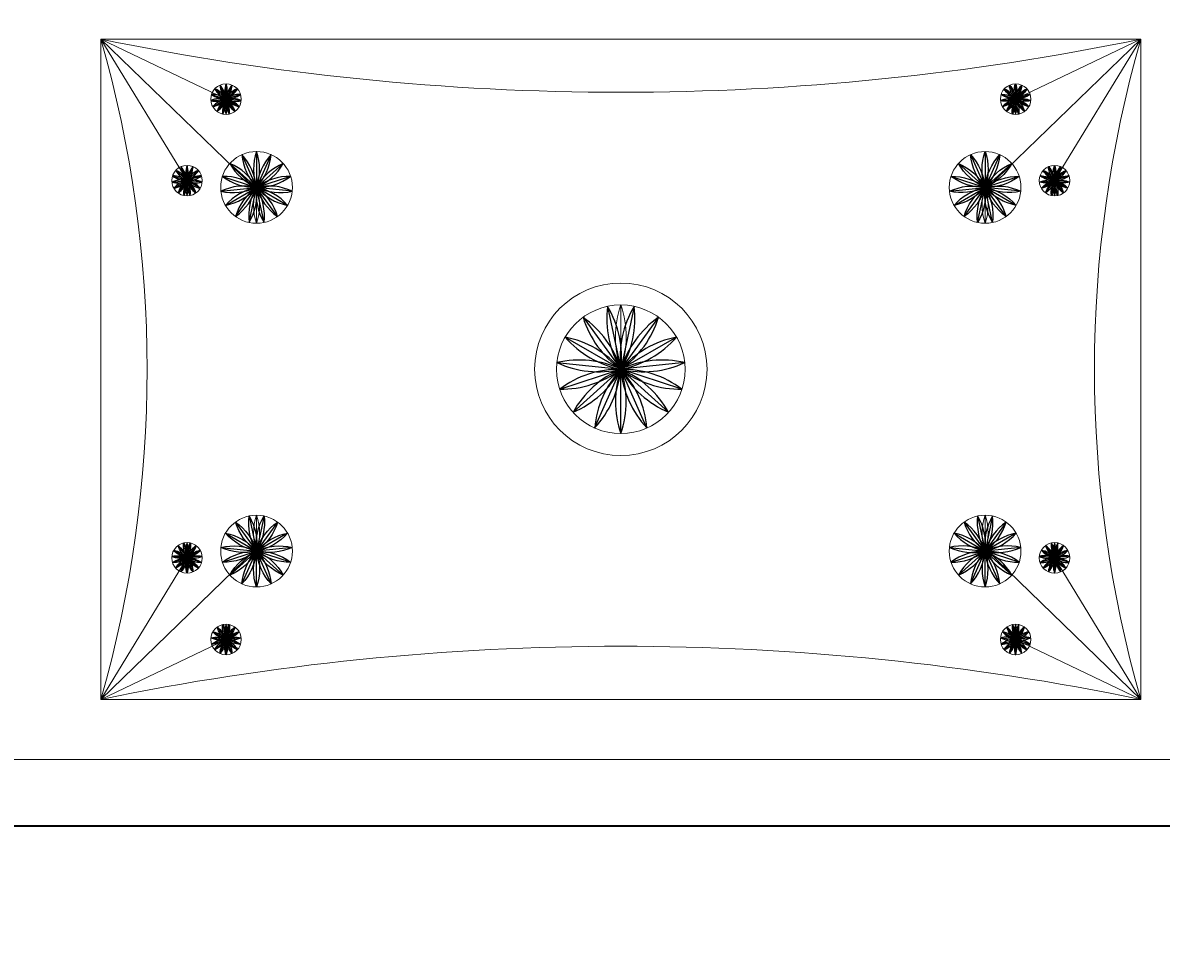
# Model space of a CAD drawing. Units: inches. Extents: x -61 to 1599, y -1316 to 257.
# Tile 117 of 204: x 134 to 161, y -10 to 11. Entities that reach past the tile are written whole.
import ezdxf

# ---------------------------------------------------------------- set-up
doc = ezdxf.new("R2010")
doc.units = ezdxf.units.IN
doc.header["$MEASUREMENT"] = 0
for name, color, linetype, lineweight in [('A-ANNO-DIMS', 2, 'Continuous', 18), ('FURNITURE', 83, 'Continuous', 18), ('WALLS', 4, 'Continuous', 35)]:
    doc.layers.add(name, color=color, linetype=linetype, lineweight=lineweight)
doc.layers.add('LT', color=8, linetype='Continuous')
doc.styles.get("Standard").update_dxf_attribs({"font": 'arial.ttf'})
doc.dimstyles.get("Standard").update_dxf_attribs({"dimtxt": 0.18, "dimasz": 0.18, "dimexe": 0.18, "dimexo": 0.0625, "dimgap": 0.09, "dimtad": 0, "dimtih": 1, "dimtoh": 1, "dimdec": 0, "dimzin": 0, "dimdsep": 46, "dimlunit": 3, "dimtxsty": 'Standard', "dimcen": 0.09, "dimadec": 0, "dimazin": 0, "dimtfac": 1, "dimtdec": 0, "dimtofl": 0, "dimtmove": 0, "dimatfit": 3, "dimfxl": 1, "dimtolj": 1, "dimtzin": 0, "dimarcsym": 0})

# ---------------------------------------------------------------- blocks, each defined once
blk = doc.blocks.new('*U3')
at = {"layer": 'LT'}
blk.add_line((0, 0.175), (0, -0.175), dxfattribs=at)
for centre, start, end in [((0.509, 0), 160.9983, 199.0017), ((-0.509, 0), 340.9983, 19.0017)]:
    blk.add_arc(centre, 0.539, start, end, dxfattribs=at)
blk = doc.blocks.new('*U4')
at = {"layer": 'LT', "transparency": 16777216}
for p, rotation in [((-66.605, -18.692), 48.00000000000001), ((-66.546, -18.649), 24), ((-66.404, -18.649), 336.0000000000001), ((-66.345, -18.692), 312), ((-66.649, -18.828), 96), ((-66.642, -18.755), 72), ((-66.627, -18.897), 120), ((-66.578, -18.951), 144), ((-66.512, -18.981), 168.0000000000001), ((-66.439, -18.981), 192), ((-66.372, -18.951), 216), ((-66.323, -18.897), 240), ((-66.308, -18.755), 288.0000000000001), ((-66.301, -18.828), 264)]:
    blk.add_blockref('*U3', p, dxfattribs=dict(at, rotation=rotation))
blk.add_blockref('*U3', (-66.475, -18.634), dxfattribs=at)
blk = doc.blocks.new('*U20')
at = {"layer": 'LT'}
blk.add_line((0, 0.175), (0, -0.175), dxfattribs=at)
for centre, start, end in [((0.509, 0), 160.9983, 199.0017), ((-0.509, 0), 340.9983, 19.0017)]:
    blk.add_arc(centre, 0.539, start, end, dxfattribs=at)
blk = doc.blocks.new('*U21')
at = {"layer": 'LT', "transparency": 16777216}
for p, rotation in [((-66.605, -18.692), 48.00000000000001), ((-66.546, -18.649), 24), ((-66.404, -18.649), 336.0000000000001), ((-66.345, -18.692), 312), ((-66.649, -18.828), 96), ((-66.642, -18.755), 72), ((-66.627, -18.897), 120), ((-66.578, -18.951), 144), ((-66.512, -18.981), 168.0000000000001), ((-66.439, -18.981), 192), ((-66.372, -18.951), 216), ((-66.323, -18.897), 240), ((-66.308, -18.755), 288.0000000000001), ((-66.301, -18.828), 264)]:
    blk.add_blockref('*U20', p, dxfattribs=dict(at, rotation=rotation))
blk.add_blockref('*U20', (-66.475, -18.634), dxfattribs=at)
blk = doc.blocks.new('*U52')
at = {"layer": 'LT'}
blk.add_line((0, 0.175), (0, -0.175), dxfattribs=at)
for centre, start, end in [((0.509, 0), 160.9983, 199.0017), ((-0.509, 0), 340.9983, 19.0017)]:
    blk.add_arc(centre, 0.539, start, end, dxfattribs=at)
blk = doc.blocks.new('*U53')
at = {"layer": 'LT', "transparency": 16777216}
for p, rotation in [((-66.605, -18.692), 48.00000000000001), ((-66.546, -18.649), 24), ((-66.404, -18.649), 336.0000000000001), ((-66.345, -18.692), 312), ((-66.649, -18.828), 96), ((-66.642, -18.755), 72), ((-66.627, -18.897), 120), ((-66.578, -18.951), 144), ((-66.512, -18.981), 168.0000000000001), ((-66.439, -18.981), 192), ((-66.372, -18.951), 216), ((-66.323, -18.897), 240), ((-66.308, -18.755), 288.0000000000001), ((-66.301, -18.828), 264)]:
    blk.add_blockref('*U52', p, dxfattribs=dict(at, rotation=rotation))
blk.add_blockref('*U52', (-66.475, -18.634), dxfattribs=at)
blk = doc.blocks.new('*U29')
at = {"layer": 'LT'}
blk.add_line((0, 0.175), (0, -0.175), dxfattribs=at)
for centre, start, end in [((0.509, 0), 160.9983, 199.0017), ((-0.509, 0), 340.9983, 19.0017)]:
    blk.add_arc(centre, 0.539, start, end, dxfattribs=at)
blk = doc.blocks.new('*U30')
at = {"layer": 'LT', "transparency": 16777216}
for p, rotation in [((-66.605, -18.692), 48.00000000000001), ((-66.546, -18.649), 24), ((-66.404, -18.649), 336.0000000000001), ((-66.345, -18.692), 312), ((-66.649, -18.828), 96), ((-66.642, -18.755), 72), ((-66.627, -18.897), 120), ((-66.578, -18.951), 144), ((-66.512, -18.981), 168.0000000000001), ((-66.439, -18.981), 192), ((-66.372, -18.951), 216), ((-66.323, -18.897), 240), ((-66.308, -18.755), 288.0000000000001), ((-66.301, -18.828), 264)]:
    blk.add_blockref('*U29', p, dxfattribs=dict(at, rotation=rotation))
blk.add_blockref('*U29', (-66.475, -18.634), dxfattribs=at)
blk = doc.blocks.new('*U5')
at = {"layer": 'LT'}
blk.add_line((0, 0.412), (0, -0.412), dxfattribs=at)
for centre, start, end in [((1.198, 0), 160.9983, 199.0017), ((-1.198, 0), 340.9983, 19.0017)]:
    blk.add_arc(centre, 1.267, start, end, dxfattribs=at)
blk = doc.blocks.new('*U47')
at = {"layer": 'LT', "transparency": 16777216}
for p, rotation in [((-156.501, -43.858), 24), ((-156.165, -43.858), 336.0000000000001), ((-156.639, -43.959), 48.00000000000001), ((-156.027, -43.959), 312), ((-156.725, -44.108), 72), ((-155.941, -44.108), 288.0000000000001), ((-156.743, -44.278), 96), ((-156.69, -44.441), 120), ((-156.575, -44.569), 144), ((-156.419, -44.639), 168), ((-156.247, -44.639), 192), ((-156.091, -44.569), 216), ((-155.976, -44.441), 240), ((-155.923, -44.278), 264)]:
    blk.add_blockref('*U5', p, dxfattribs=dict(at, rotation=rotation))
blk.add_blockref('*U5', (-156.333, -43.823), dxfattribs=at)
blk = doc.blocks.new('*U22')
at = {"layer": 'LT'}
blk.add_line((0, 0.412), (0, -0.412), dxfattribs=at)
for centre, start, end in [((1.198, 0), 160.9983, 199.0017), ((-1.198, 0), 340.9983, 19.0017)]:
    blk.add_arc(centre, 1.267, start, end, dxfattribs=at)
blk = doc.blocks.new('*U23')
at = {"layer": 'LT', "transparency": 16777216}
for p, rotation in [((-156.501, -43.858), 24), ((-156.165, -43.858), 336.0000000000001), ((-156.639, -43.959), 48.00000000000001), ((-156.027, -43.959), 312), ((-156.725, -44.108), 72), ((-155.941, -44.108), 288.0000000000001), ((-156.743, -44.278), 96), ((-156.69, -44.441), 120), ((-156.575, -44.569), 144), ((-156.419, -44.639), 168), ((-156.247, -44.639), 192), ((-156.091, -44.569), 216), ((-155.976, -44.441), 240), ((-155.923, -44.278), 264)]:
    blk.add_blockref('*U22', p, dxfattribs=dict(at, rotation=rotation))
blk.add_blockref('*U22', (-156.333, -43.823), dxfattribs=at)
blk = doc.blocks.new('*U54')
at = {"layer": 'LT'}
blk.add_line((0, 0.739), (0, -0.739), dxfattribs=at)
for centre, start, end in [((2.147, 0), 160.9983, 199.0017), ((-2.147, 0), 340.9983, 19.0017)]:
    blk.add_arc(centre, 2.27, start, end, dxfattribs=at)
blk = doc.blocks.new('*U41')
at = {"layer": 'LT', "transparency": 16777216}
for p, rotation in [((-280.542, -78.621), 23.99999999999999), ((-279.941, -78.621), 336.0000000000001), ((-280.791, -78.801), 48.00000000000001), ((-279.692, -78.801), 312), ((-280.945, -79.067), 72), ((-279.539, -79.067), 288.0000000000001), ((-280.977, -79.373), 96), ((-280.882, -79.665), 120), ((-280.676, -79.894), 144), ((-280.395, -80.019), 168), ((-280.088, -80.019), 191.9999999999999), ((-279.807, -79.894), 216), ((-279.602, -79.665), 240), ((-279.507, -79.373), 264)]:
    blk.add_blockref('*U54', p, dxfattribs=dict(at, rotation=rotation))
blk.add_blockref('*U54', (-280.242, -78.557), dxfattribs=at)
blk = doc.blocks.new('*U42')
at = {"layer": 'LT'}
blk.add_line((0, 0.412), (0, -0.412), dxfattribs=at)
for centre, start, end in [((1.198, 0), 160.9983, 199.0017), ((-1.198, 0), 340.9983, 19.0017)]:
    blk.add_arc(centre, 1.267, start, end, dxfattribs=at)
blk = doc.blocks.new('*U43')
at = {"layer": 'LT', "transparency": 16777216}
for p, rotation in [((-156.501, -43.858), 24), ((-156.165, -43.858), 336.0000000000001), ((-156.639, -43.959), 48.00000000000001), ((-156.027, -43.959), 312), ((-156.725, -44.108), 72), ((-155.941, -44.108), 288.0000000000001), ((-156.743, -44.278), 96), ((-156.69, -44.441), 120), ((-156.575, -44.569), 144), ((-156.419, -44.639), 168), ((-156.247, -44.639), 192), ((-156.091, -44.569), 216), ((-155.976, -44.441), 240), ((-155.923, -44.278), 264)]:
    blk.add_blockref('*U42', p, dxfattribs=dict(at, rotation=rotation))
blk.add_blockref('*U42', (-156.333, -43.823), dxfattribs=at)
blk = doc.blocks.new('*U31')
at = {"layer": 'LT'}
blk.add_line((0, 0.412), (0, -0.412), dxfattribs=at)
for centre, start, end in [((1.198, 0), 160.9983, 199.0017), ((-1.198, 0), 340.9983, 19.0017)]:
    blk.add_arc(centre, 1.267, start, end, dxfattribs=at)
blk = doc.blocks.new('*U32')
at = {"layer": 'LT', "transparency": 16777216}
for p, rotation in [((-156.501, -43.858), 24), ((-156.165, -43.858), 336.0000000000001), ((-156.639, -43.959), 48.00000000000001), ((-156.027, -43.959), 312), ((-156.725, -44.108), 72), ((-155.941, -44.108), 288.0000000000001), ((-156.743, -44.278), 96), ((-156.69, -44.441), 120), ((-156.575, -44.569), 144), ((-156.419, -44.639), 168), ((-156.247, -44.639), 192), ((-156.091, -44.569), 216), ((-155.976, -44.441), 240), ((-155.923, -44.278), 264)]:
    blk.add_blockref('*U31', p, dxfattribs=dict(at, rotation=rotation))
blk.add_blockref('*U31', (-156.333, -43.823), dxfattribs=at)
blk = doc.blocks.new('*U48')
at = {"layer": 'LT'}
blk.add_line((0, 0.175), (0, -0.175), dxfattribs=at)
for centre, start, end in [((0.509, 0), 160.9983, 199.0017), ((-0.509, 0), 340.9983, 19.0017)]:
    blk.add_arc(centre, 0.539, start, end, dxfattribs=at)
blk = doc.blocks.new('*U49')
at = {"layer": 'LT', "transparency": 16777216}
for p, rotation in [((-66.605, -18.692), 48.00000000000001), ((-66.546, -18.649), 24), ((-66.404, -18.649), 336.0000000000001), ((-66.345, -18.692), 312), ((-66.649, -18.828), 96), ((-66.642, -18.755), 72), ((-66.627, -18.897), 120), ((-66.578, -18.951), 144), ((-66.512, -18.981), 168.0000000000001), ((-66.439, -18.981), 192), ((-66.372, -18.951), 216), ((-66.323, -18.897), 240), ((-66.308, -18.755), 288.0000000000001), ((-66.301, -18.828), 264)]:
    blk.add_blockref('*U48', p, dxfattribs=dict(at, rotation=rotation))
blk.add_blockref('*U48', (-66.475, -18.634), dxfattribs=at)
blk = doc.blocks.new('*U24')
at = {"layer": 'LT'}
blk.add_line((0, 0.175), (0, -0.175), dxfattribs=at)
for centre, start, end in [((0.509, 0), 160.9983, 199.0017), ((-0.509, 0), 340.9983, 19.0017)]:
    blk.add_arc(centre, 0.539, start, end, dxfattribs=at)
blk = doc.blocks.new('*U25')
at = {"layer": 'LT', "transparency": 16777216}
for p, rotation in [((-66.605, -18.692), 48.00000000000001), ((-66.546, -18.649), 24), ((-66.404, -18.649), 336.0000000000001), ((-66.345, -18.692), 312), ((-66.649, -18.828), 96), ((-66.642, -18.755), 72), ((-66.627, -18.897), 120), ((-66.578, -18.951), 144), ((-66.512, -18.981), 168.0000000000001), ((-66.439, -18.981), 192), ((-66.372, -18.951), 216), ((-66.323, -18.897), 240), ((-66.308, -18.755), 288.0000000000001), ((-66.301, -18.828), 264)]:
    blk.add_blockref('*U24', p, dxfattribs=dict(at, rotation=rotation))
blk.add_blockref('*U24', (-66.475, -18.634), dxfattribs=at)
blk = doc.blocks.new('*U50')
at = {"layer": 'LT'}
blk.add_line((0, 0.175), (0, -0.175), dxfattribs=at)
for centre, start, end in [((0.509, 0), 160.9983, 199.0017), ((-0.509, 0), 340.9983, 19.0017)]:
    blk.add_arc(centre, 0.539, start, end, dxfattribs=at)
blk = doc.blocks.new('*U51')
at = {"layer": 'LT', "transparency": 16777216}
for p, rotation in [((-66.605, -18.692), 48.00000000000001), ((-66.546, -18.649), 24), ((-66.404, -18.649), 336.0000000000001), ((-66.345, -18.692), 312), ((-66.649, -18.828), 96), ((-66.642, -18.755), 72), ((-66.627, -18.897), 120), ((-66.578, -18.951), 144), ((-66.512, -18.981), 168.0000000000001), ((-66.439, -18.981), 192), ((-66.372, -18.951), 216), ((-66.323, -18.897), 240), ((-66.308, -18.755), 288.0000000000001), ((-66.301, -18.828), 264)]:
    blk.add_blockref('*U50', p, dxfattribs=dict(at, rotation=rotation))
blk.add_blockref('*U50', (-66.475, -18.634), dxfattribs=at)
blk = doc.blocks.new('*U26')
at = {"layer": 'LT'}
blk.add_line((0, 0.175), (0, -0.175), dxfattribs=at)
for centre, start, end in [((0.509, 0), 160.9983, 199.0017), ((-0.509, 0), 340.9983, 19.0017)]:
    blk.add_arc(centre, 0.539, start, end, dxfattribs=at)
blk = doc.blocks.new('*U27')
at = {"layer": 'LT', "transparency": 16777216}
for p, rotation in [((-66.605, -18.692), 48.00000000000001), ((-66.546, -18.649), 24), ((-66.404, -18.649), 336.0000000000001), ((-66.345, -18.692), 312), ((-66.649, -18.828), 96), ((-66.642, -18.755), 72), ((-66.627, -18.897), 120), ((-66.578, -18.951), 144), ((-66.512, -18.981), 168.0000000000001), ((-66.439, -18.981), 192), ((-66.372, -18.951), 216), ((-66.323, -18.897), 240), ((-66.308, -18.755), 288.0000000000001), ((-66.301, -18.828), 264)]:
    blk.add_blockref('*U26', p, dxfattribs=dict(at, rotation=rotation))
blk.add_blockref('*U26', (-66.475, -18.634), dxfattribs=at)
blk = doc.blocks.new('BED-DOUBLE')
for p, q in [((37.147, 1.379), (37.147, 16.557)), ((61.064, 16.557), (37.147, 16.557)), ((37.147, 16.557), (40.027, 15.18)), ((37.147, 16.557), (40.715, 13.107)), ((37.147, 16.557), (39.13, 13.305)), ((61.064, 16.557), (57.496, 13.107)), ((61.064, 16.557), (58.185, 15.18)), ((61.064, 16.557), (59.081, 13.305)), ((40.027, 15.18), (40.027, 14.829)), ((58.185, 15.18), (58.185, 14.829)), ((39.13, 13.305), (39.13, 12.955)), ((40.729, 13.149), (40.729, 12.324)), ((57.483, 13.149), (57.483, 12.324)), ((59.081, 13.305), (59.081, 12.955)), ((49.106, 8.968), (49.106, 10.447)), ((40.729, 4.788), (40.729, 5.613)), ((57.483, 4.788), (57.483, 5.613)), ((39.13, 4.631), (39.13, 4.982)), ((59.081, 4.631), (59.081, 4.982)), ((37.147, 1.379), (40.715, 4.83)), ((61.064, 1.379), (57.496, 4.83)), ((37.147, 1.379), (39.13, 4.631)), ((61.064, 1.379), (59.081, 4.631)), ((40.027, 2.756), (40.027, 3.107)), ((58.185, 2.756), (58.185, 3.107)), ((37.147, 1.379), (40.027, 2.756)), ((61.064, 1.379), (58.185, 2.756)), ((61.064, 1.379), (61.064, 1.379))]:
    blk.add_line(p, q)
for points in [[(1.272, 88.537), (1.272, 3.449, 0.414214), (4.722, 0), (66.813, 0, 0.414214), (70.263, 3.449), (70.263, 88.537, 0.414214), (66.813, 91.987), (4.722, 91.987, 0.414214)], [(40.027, 15.18, 0.167358), (40.027, 14.829, 0.167358)], [(39.13, 13.305, 0.167358), (39.13, 12.955, 0.167358)], [(40.729, 13.149, 0.167358), (40.729, 12.324, 0.167358)], [(57.483, 12.324, 0.167358), (57.483, 13.149, 0.167358)], [(59.081, 12.955, 0.167358), (59.081, 13.305, 0.167358)], [(49.106, 8.968, 0.167358), (49.106, 10.447, 0.167358)], [(40.729, 5.613, 0.167358), (40.729, 4.788, 0.167358)], [(57.483, 4.788, 0.167358), (57.483, 5.613, 0.167358)], [(39.13, 4.982, 0.167358), (39.13, 4.631, 0.167358)], [(59.081, 4.631, 0.167358), (59.081, 4.982, 0.167358)], [(40.027, 3.107, 0.167358), (40.027, 2.756, 0.167358)], [(58.185, 2.756, 0.167358), (58.185, 3.107, 0.167358)]]:
    blk.add_lwpolyline(points, format="xyb", close=True)
blk.add_lwpolyline([(61.064, 16.557), (61.064, 1.379), (37.147, 1.379)])
for centre, radius in [((40.027, 15.18), 0.351), ((58.185, 15.18), 0.351), ((40.729, 13.149), 0.825), ((57.483, 13.149), 0.825), ((39.13, 13.305), 0.351), ((59.081, 13.305), 0.351), ((49.106, 8.968), 1.982), ((49.106, 8.968), 1.478), ((40.729, 4.788), 0.825), ((57.483, 4.788), 0.825), ((39.13, 4.631), 0.351), ((59.081, 4.631), 0.351), ((40.027, 2.756), 0.351), ((58.185, 2.756), 0.351)]:
    blk.add_circle(centre, radius)
for centre, radius, start, end in [((10.674, 8.968), 27.54, 344.0046, 15.9954), ((49.106, 74.54), 59.203, 258.34678, 281.65322), ((87.538, 8.968), 27.54, 164.0046, 195.9954), ((58.694, 15.005), 0.539, 160.9983, 199.0017), ((57.675, 15.005), 0.539, 340.9983, 19.0017), ((49.106, -56.603), 59.203, 78.34678, 101.65322)]:
    blk.add_arc(centre, radius, start, end)
for name, p in [('*U30', (106.502, 33.99)), ('*U23', (197.062, 57.384)), ('*U21', (105.605, 32.115))]:
    blk.add_blockref(name, p)
at = {"extrusion": (0, 0, -1), "zscale": -1}
for name, p in [('*U25', (8.291, 33.99)), ('*U32', (98.85, 57.384)), ('*U27', (7.394, 32.115))]:
    blk.add_blockref(name, p, dxfattribs=at)
at = {"rotation": 180}
for name, p in [('*U41', (-231.136, -70.328)), ('*U43', (-98.85, -39.447)), ('*U51', (-7.394, -14.178)), ('*U49', (-8.291, -16.053))]:
    blk.add_blockref(name, p, dxfattribs=at)
at = {"extrusion": (0, 0, -1), "zscale": -1, "rotation": 180}
for name, p in [('*U47', (-197.062, -39.447)), ('*U4', (-105.605, -14.178)), ('*U53', (-106.502, -16.053))]:
    blk.add_blockref(name, p, dxfattribs=at)
blk = doc.blocks.new('*D687')
at = {"layer": 'A-ANNO-DIMS', "color": 0, "lineweight": -2, "transparency": 16777216}
for p, q in [((289.418, 181.677), (-61.077, 181.677)), ((-60.897, 181.497), (-60.897, -528.952)), ((-60.897, -1239.765), (-60.897, -529.316)), ((319.64, -1239.945), (-61.077, -1239.945))]:
    blk.add_line(p, q, dxfattribs=at)
at = {"layer": 'A-ANNO-DIMS', "color": 0, "transparency": 16777216}
for points in [[(-60.927, 181.497), (-60.867, 181.497), (-60.897, 181.677)], [(-60.927, -1239.765), (-60.867, -1239.765), (-60.897, -1239.945)]]:
    blk.add_solid(points, dxfattribs=at)
at = {"layer": 'DEFPOINTS', "color": 0, "transparency": 16777216}
for p in [(289.481, 181.677), (-60.897, -1239.945), (319.703, -1239.945)]:
    blk.add_point(p, dxfattribs=at)
at = {"layer": 'A-ANNO-DIMS', "color": 0, "transparency": 16777216, "insert": (-60.897, -529.134), "char_height": 0.18, "attachment_point": 5}
blk.add_mtext('\\A1;1421.6', dxfattribs=at)
blk = doc.blocks.new('*D700')
at = {"layer": 'A-ANNO-DIMS', "color": 0, "lineweight": -2, "transparency": 16777216}
for p, q in [((14.703, -616.882), (14.703, 257.457)), ((179.752, -616.882), (179.752, 257.457)), ((14.883, 257.277), (96.772, 257.277)), ((179.572, 257.277), (97.683, 257.277))]:
    blk.add_line(p, q, dxfattribs=at)
at = {"layer": 'A-ANNO-DIMS', "color": 0, "transparency": 16777216}
for points in [[(14.883, 257.307), (14.883, 257.247), (14.703, 257.277)], [(179.572, 257.307), (179.572, 257.247), (179.752, 257.277)]]:
    blk.add_solid(points, dxfattribs=at)
at = {"layer": 'DEFPOINTS', "color": 0, "transparency": 16777216}
for p in [(179.752, 257.277), (14.703, -616.945), (179.752, -616.945)]:
    blk.add_point(p, dxfattribs=at)
at = {"layer": 'A-ANNO-DIMS', "color": 0, "transparency": 16777216, "insert": (97.227, 257.277), "char_height": 0.18, "attachment_point": 5}
blk.add_mtext('\\A1;165.05', dxfattribs=at)

msp = doc.modelspace()

# ---------------------------------------------------------------- linework, layer by layer
at = {"layer": 'WALLS'}
msp.add_line((87.7028, -7.3229), (185.2611, -7.3229), dxfattribs=at)

# ---------------------------------------------------------------- block references
at = {"layer": 'FURNITURE'}
msp.add_blockref('BED-DOUBLE', (98.977, -5.797), dxfattribs=at)

# ---------------------------------------------------------------- dimensions: what is measured, and where the dimension line sits
at = {"layer": 'A-ANNO-DIMS'}
dim = msp.add_linear_dim(base=(179.7521, 257.2771), p1=(14.7028, -616.9446), p2=(179.7521, -616.9446), dimstyle='Standard', override={"dimdec": 2, "dimlfac": 1, "dimrnd": 0, "dimzin": 0, "dimdsep": 46, "dimlunit": 2}, dxfattribs=at)
dim.commit()
dim.dimension.update_dxf_attribs({"geometry": '*D700', "text_midpoint": (97.2274, 257.2771)})
dim = msp.add_linear_dim(base=(-60.8972, -1239.9446), p1=(289.4807, 181.6771), p2=(319.7028, -1239.9446), angle=90, dimstyle='Standard', override={"dimdec": 1, "dimlfac": 1, "dimrnd": 0, "dimzin": 0, "dimdsep": 46, "dimlunit": 2}, dxfattribs=at)
dim.commit()
dim.dimension.update_dxf_attribs({"geometry": '*D687', "text_midpoint": (-60.8972, -529.1337)})

doc.saveas('drawing.dxf')
